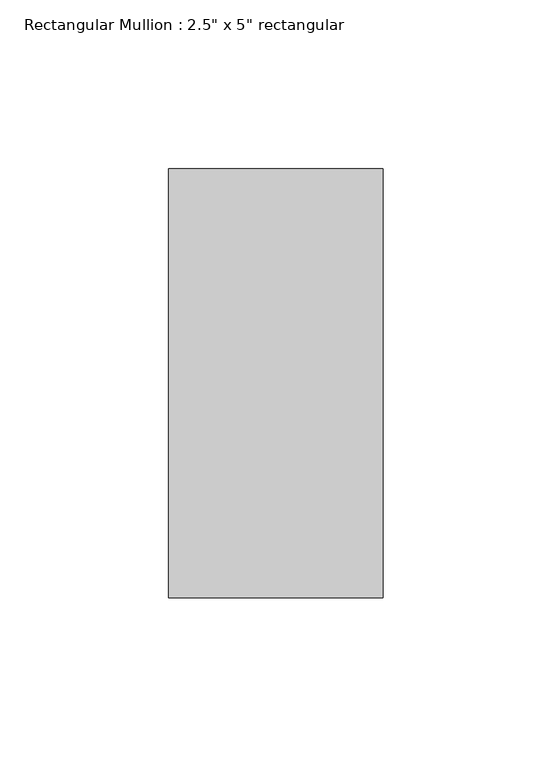
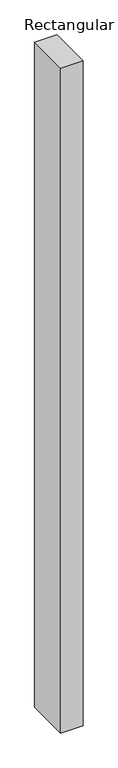
"""IFC4 building model written with IfcOpenShell, lengths in millimetres: member geometry."""

from ifc_helpers import new_model, si_unit, frame, origin, place, context, project, spatial, polyline, outline, extrude, source, transform, mapped, element, save


def member_dae9f1c3(model_context):
    return source(origin(), model_context, "Body", "SweptSolid", [
        extrude(outline(polyline([(0.0, 63.5), (0.0, -63.5), (-63.5, -63.5), (-63.5, 63.5), (0.0, 63.5)])), frame((0.0, 0.0, -1988.699716), z_axis=(0.0, 0.0, 1.0), x_axis=(1.0, 0.0, 0.0)), (0.0, 0.0, 1.0), 1988.699716),
    ])


if __name__ == "__main__":
    model = new_model("IFC4")
    model_context = context("Model", 3, world=origin())
    ifc_project = project(units=[si_unit("LENGTHUNIT", "METRE", prefix="MILLI")], contexts=[model_context])
    site = spatial("IfcSite", under=ifc_project)
    building = spatial("IfcBuilding", under=site)
    placement = place(None, origin())
    member_shape = member_dae9f1c3(model_context)
    element("IfcMember", 1, ObjectType="Rectangular Mullion : 2.5\" x 5\" rectangular", at=placement, inside=building, context=model_context, shape_type="MappedRepresentation", body=[
        mapped(member_shape, transform((0.0, 0.0, 0.0), x_axis=(1.0, 0.0, 0.0), y_axis=(0.0, 1.0, 0.0), z_axis=(0.0, 0.0, 1.0))),
    ])
    save(model, "model.ifc")

# Revit data of these elements
# Type "Rectangular Mullion : 2.5\" x 5\" rectangular"
#   built-in parameter 1007304 = 0.416667 (stored number, unit not read)
#   built-in parameter 1007301 = 0.104167 (stored number, unit not read)
#   built-in parameter 1007300 = 0.104167 (stored number, unit not read)
# Element 1 (IfcMember, "Rectangular Mullion : 2.5\" x 5\" rectangular")
#   Materials on its faces: "Aluminum"
# Materials
#   "Aluminum": class "Metal", colour RGB 247 247 247, transparency 0, Description = "Aluminum 6061", Cost = 0
